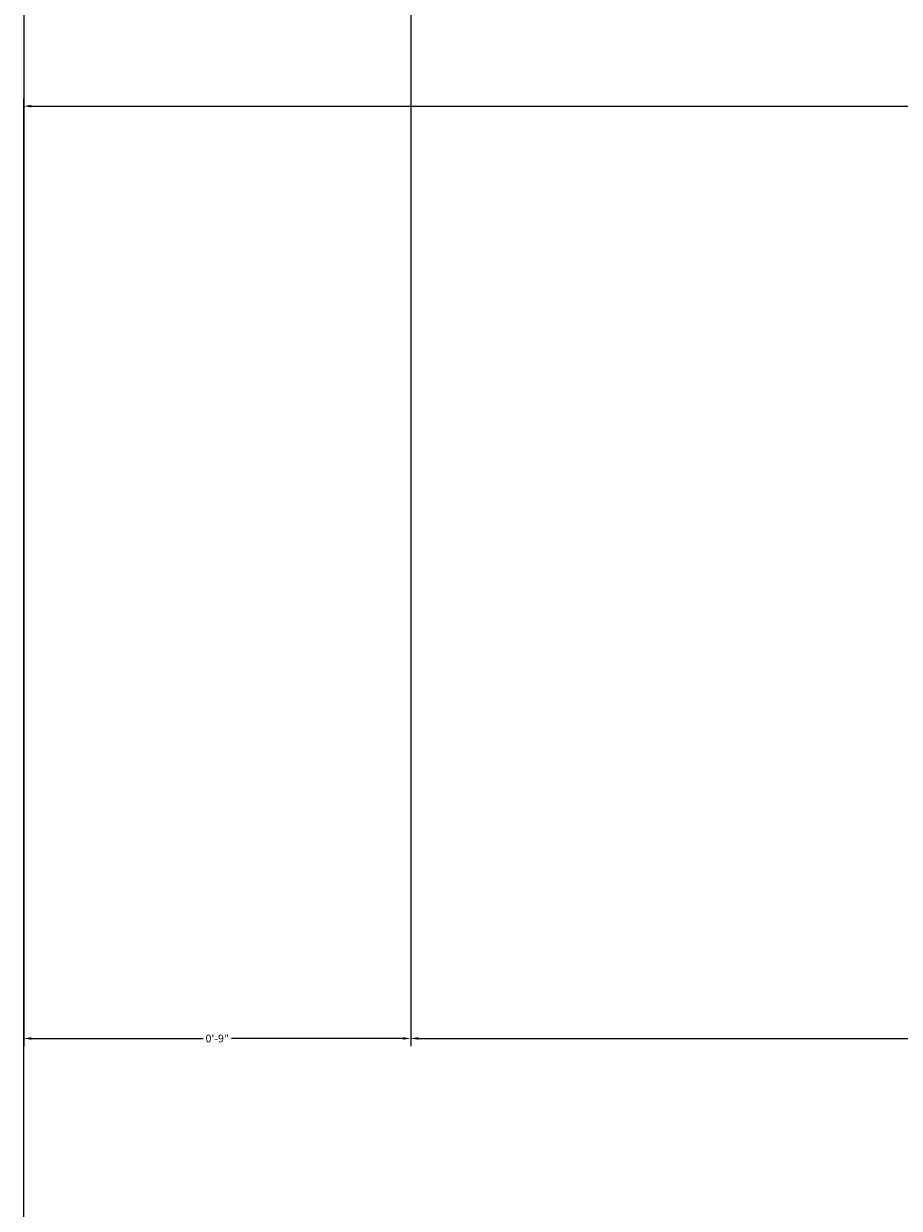
# Model space of a CAD drawing. Units: inches. Extents: x 37 to 824, y -700 to 234.
# Tile 7 of 77: x 161 to 181, y -404 to -377. Entities that reach past the tile are written whole.
import ezdxf

# ---------------------------------------------------------------- set-up
doc = ezdxf.new("R2010")
doc.units = ezdxf.units.IN
doc.header["$MEASUREMENT"] = 0
doc.layers.add('A-ANNO-DIMS', color=2, linetype='Continuous', lineweight=18)
doc.styles.get("Standard").update_dxf_attribs({"font": 'arial.ttf'})
doc.dimstyles.get("Standard").update_dxf_attribs({"dimtxt": 0.18, "dimasz": 0.18, "dimexe": 0.18, "dimexo": 0.0625, "dimgap": 0.09, "dimtad": 0, "dimtih": 1, "dimtoh": 1, "dimdec": 1, "dimzin": 0, "dimdsep": 46, "dimlunit": 4, "dimtxsty": 'Standard', "dimcen": 0.09, "dimadec": 0, "dimazin": 0, "dimtfac": 1, "dimtdec": 1, "dimtofl": 0, "dimtmove": 0, "dimatfit": 3, "dimfxl": 1, "dimtolj": 1, "dimtzin": 0, "dimarcsym": 0})

# ---------------------------------------------------------------- blocks, each defined once
blk = doc.blocks.new('*D66')
at = {"layer": 'A-ANNO-DIMS', "color": 0, "lineweight": -2, "ltscale": 0.5, "transparency": 16777216}
for p, q in [((161.077, -423.565), (161.077, -378.38)), ((428.077, -423.565), (428.077, -378.38)), ((161.257, -378.56), (294.176, -378.56)), ((427.897, -378.56), (294.978, -378.56))]:
    blk.add_line(p, q, dxfattribs=at)
at = {"layer": 'A-ANNO-DIMS', "color": 0, "ltscale": 0.5, "transparency": 16777216}
for points in [[(161.257, -378.53), (161.257, -378.59), (161.077, -378.56)], [(427.897, -378.53), (427.897, -378.59), (428.077, -378.56)]]:
    blk.add_solid(points, dxfattribs=at)
at = {"layer": 'Defpoints', "color": 0, "ltscale": 0.5, "transparency": 16777216}
for p in [(428.077, -378.56), (161.077, -423.627), (428.077, -423.627)]:
    blk.add_point(p, dxfattribs=at)
at = {"layer": 'A-ANNO-DIMS', "color": 0, "ltscale": 0.5, "transparency": 16777216, "insert": (294.577, -378.56), "char_height": 0.18, "attachment_point": 5}
blk.add_mtext('\\A1;22\'-3"', dxfattribs=at)
blk = doc.blocks.new('*D80')
at = {"layer": 'A-ANNO-DIMS', "color": 0, "lineweight": -2, "ltscale": 0.5, "transparency": 16777216}
for p, q in [((170.077, -167.972), (170.077, -400.406)), ((250.19, -167.972), (250.19, -400.406)), ((170.257, -400.226), (209.804, -400.226)), ((250.01, -400.226), (210.463, -400.226))]:
    blk.add_line(p, q, dxfattribs=at)
at = {"layer": 'A-ANNO-DIMS', "color": 0, "ltscale": 0.5, "transparency": 16777216}
for points in [[(170.257, -400.196), (170.257, -400.256), (170.077, -400.226)], [(250.01, -400.196), (250.01, -400.256), (250.19, -400.226)]]:
    blk.add_solid(points, dxfattribs=at)
at = {"layer": 'Defpoints', "color": 0, "ltscale": 0.5, "transparency": 16777216}
for p in [(170.077, -167.91), (250.19, -167.91), (250.19, -400.226)]:
    blk.add_point(p, dxfattribs=at)
at = {"layer": 'A-ANNO-DIMS', "color": 0, "ltscale": 0.5, "transparency": 16777216, "insert": (210.133, -400.226), "char_height": 0.18, "attachment_point": 5}
blk.add_mtext('\\A1;6\'-8"', dxfattribs=at)
blk = doc.blocks.new('*D89')
at = {"layer": 'A-ANNO-DIMS', "color": 0, "lineweight": -2, "ltscale": 0.5, "transparency": 16777216}
for p, q in [((170.077, -356.972), (170.077, -400.406)), ((161.077, -365.972), (161.077, -400.406)), ((161.257, -400.226), (165.248, -400.226)), ((169.897, -400.226), (165.906, -400.226))]:
    blk.add_line(p, q, dxfattribs=at)
at = {"layer": 'A-ANNO-DIMS', "color": 0, "ltscale": 0.5, "transparency": 16777216}
for points in [[(161.257, -400.196), (161.257, -400.256), (161.077, -400.226)], [(169.897, -400.196), (169.897, -400.256), (170.077, -400.226)]]:
    blk.add_solid(points, dxfattribs=at)
at = {"layer": 'Defpoints', "color": 0, "ltscale": 0.5, "transparency": 16777216}
for p in [(170.077, -356.91), (161.077, -365.91), (170.077, -400.226)]:
    blk.add_point(p, dxfattribs=at)
at = {"layer": 'A-ANNO-DIMS', "color": 0, "ltscale": 0.5, "transparency": 16777216, "insert": (165.577, -400.226), "char_height": 0.18, "attachment_point": 5}
blk.add_mtext('\\A1;0\'-9"', dxfattribs=at)

msp = doc.modelspace()

# ---------------------------------------------------------------- dimensions: what is measured, and where the dimension line sits
at = {"layer": 'A-ANNO-DIMS', "ltscale": 0.5}
for base, p1, p2, picture, middle in [((250.19, -400.226), (170.077, -167.91), (250.19, -167.91), '*D80', (210.133, -400.226)), ((170.077, -400.226), (161.077, -365.91), (170.077, -356.91), '*D89', (165.577, -400.226)), ((428.077, -378.56), (161.077, -423.627), (428.077, -423.627), '*D66', (294.577, -378.56))]:
    dim = msp.add_linear_dim(base=base, p1=p1, p2=p2, dimstyle='Standard', override={"dimdec": 1, "dimlfac": 1, "dimrnd": 0, "dimzin": 1, "dimdsep": 46, "dimlunit": 4, "dimfrac": 2}, dxfattribs=at)
    dim.commit()
    dim.dimension.update_dxf_attribs({"geometry": picture, "text_midpoint": middle})

doc.saveas('drawing.dxf')
